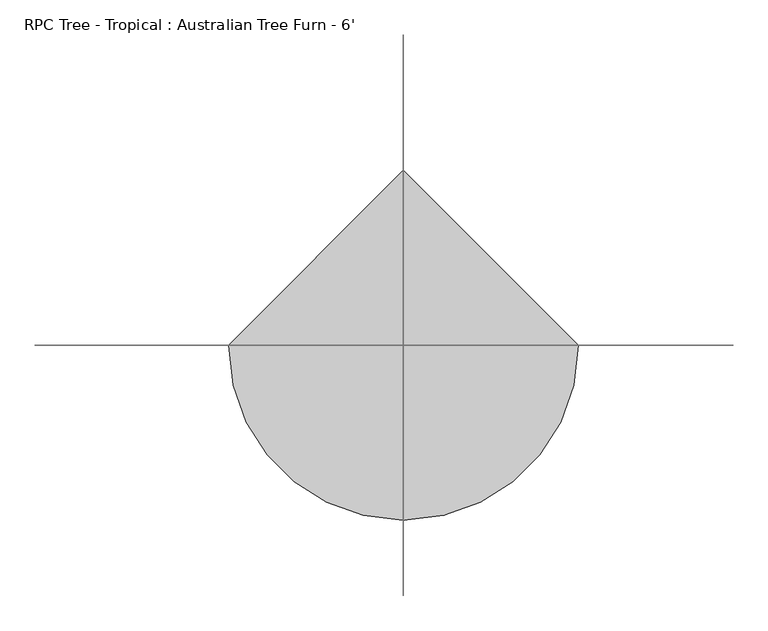
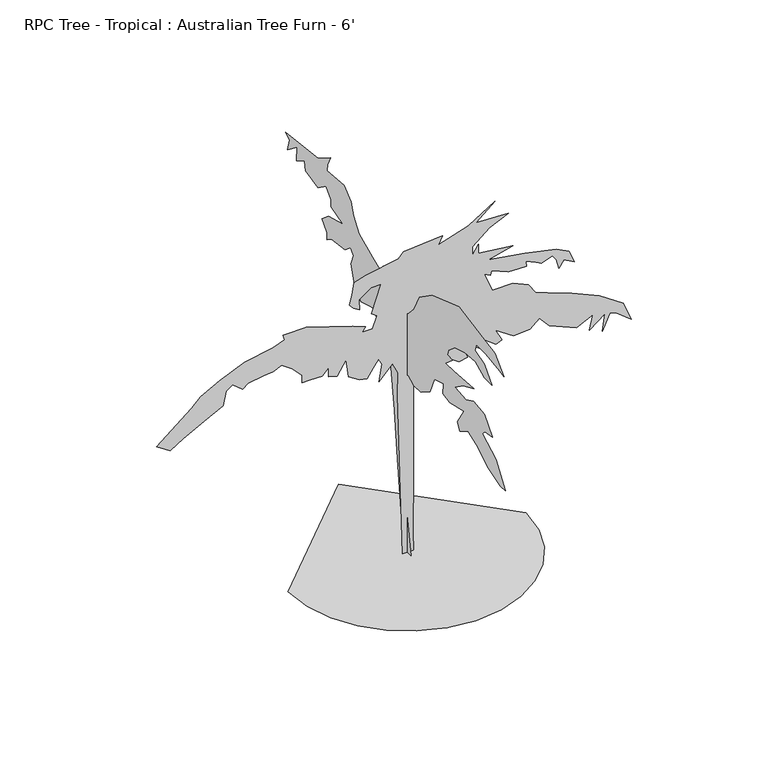
"""IFC4 building model written with IfcOpenShell, lengths in millimetres: geographic element geometry, RPC Tree - Tropical : Australian Tree Furn - 6'."""

from ifc_helpers import new_model, si_unit, origin, place, context, project, spatial, triangles, source, transform, mapped, element, save


def rpc_tree_tropical_australian_tree_furn_6_77f1a640(model_context):
    return source(origin(), model_context, "Body", "Tessellation", [
        triangles([(-639.0365753, 0.0, 0.0007159), (-622.1405136, -146.4247652, 0.0007159), (-574.0277527, -280.8912123, 0.0007159), (-498.5465315, -399.5499215, 0.0007159), (-399.5499215, -498.5465315, 0.0007159), (-280.8912123, -574.0277527, 0.0007159), (-146.4247652, -622.1405136, 0.0007159), (2.79e-05, -639.0365753, 0.0007159), (146.4247652, -622.1429844, 0.0007159), (280.8912123, -574.0277527, 0.0007159), (399.5499215, -498.5465315, 0.0007159), (498.5465315, -399.5499215, 0.0007159), (574.0277527, -280.8912123, 0.0007159), (622.1405136, -146.4247652, 0.0007159), (639.0365753, 5.59e-05, 0.0007159), (-8.38e-05, 639.0365753, 0.0007159), (470.2991641, -3.5e-05, 1828.8014534), (368.5593713, -2.98e-05, 1741.5955845), (542.9711454, -2.94e-05, 1734.3285862), (441.231389, -2.66e-05, 1687.0922253), (350.3907492, -2.2e-05, 1610.7880165), (350.3907492, -1.92e-05, 1563.5516556), (383.0932589, -2.22e-05, 1614.4202076), (383.0932589, -1.92e-05, 1563.5516556), (568.4067295, -1.79e-05, 1541.750806), (437.5966181, -1.59e-05, 1509.0482964), (633.8092781, -1.4e-05, 1476.3456413), (800.9540903, -1.18e-05, 1440.0109406), (869.9913008, -9.7e-06, 1403.673769), (899.0591486, -5.5e-06, 1334.6364132), (840.9235256, -7.5e-06, 1367.3389229), (815.4879416, -5.1e-06, 1327.3695602), (800.9540903, -8.4e-06, 1381.8729195), (779.1532408, -1.01e-05, 1410.9406219), (721.015147, -8.8e-06, 1389.1397724), (691.9473719, -9.7e-06, 1403.673769), (637.4440126, -1.12e-05, 1429.1092804), (641.0762037, -9.4e-06, 1400.0414326), (597.4745047, -9.4e-06, 1400.0414326), (542.9711454, -9.7e-06, 1403.673769), (452.1330491, -1.18e-05, 1440.0109406), (448.4983146, -1.03e-05, 1414.5754292), (415.7958049, -1.14e-05, 1432.7440876), (459.4000111, -5.1e-06, 1327.3695602), (568.4067295, -5.1e-06, 1327.3695602), (651.9778639, -2.9e-06, 1291.0347141), (688.3126373, 3e-07, 1236.5313549), (753.7176567, 1.8e-06, 1211.0958435), (884.5252247, 4.9e-06, 1160.2246754), (1033.5014511, 8.7e-06, 1094.8221268), (1160.6767553, 1.39e-05, 1007.6162579), (1204.2784544, 2.02e-05, 902.2417305), (1120.70732, 1.63e-05, 967.6468225), (1088.0048103, 1.59e-05, 974.9137482), (1048.0353024, 2.11e-05, 887.7078793), (1062.5692263, 1.55e-05, 982.1806738), (978.9980919, 1.94e-05, 916.7781979), (997.1666777, 1.44e-05, 1000.3493322), (909.9608088, 1.7e-05, 956.7450897), (764.6193169, 1.33e-05, 1018.5179907), (710.1159576, 9.6e-06, 1080.2882755), (659.2448622, 1.22e-05, 1036.684033), (572.0389206, 1.26e-05, 1029.4171074), (473.9338986, 8.7e-06, 1094.8221268), (510.2686357, 1.26e-05, 1029.4171074), (477.5660897, 1.35e-05, 1014.8831835), (324.9577085, 6.6e-06, 1131.1569002), (419.4305394, 1.44e-05, 1000.3493322), (284.9882369, 8.7e-06, 1094.8221268), (324.9577085, 1.48e-05, 993.0824066), (277.7212749, 1.52e-05, 985.8154083), (190.5151335, 1.16e-05, 1047.5857658), (88.7756132, 9.6e-06, 1080.2882755), (194.1488688, 1.52e-05, 985.8154083), (30.6385209, 1.11e-05, 1054.8526915), (34.2719928, 1.57e-05, 978.5484827), (34.2719928, 3.32e-05, 684.2282936), (34.2719928, 4.84e-05, 429.8801196), (30.6385209, 6.77e-05, 106.4923825), (34.2719928, 7.35e-05, 0.0013276), (-23.8650472, 7.39e-05, 0.0007003), (-52.9336422, 1.98e-05, 909.5111996), (-49.2999159, 1.22e-05, 1036.684033), (-78.3684632, 8.5e-06, 1098.4543905), (-151.0396997, 1.31e-05, 1022.1501818), (-136.5055487, 7.5e-06, 1116.6229763), (-154.6734259, 5.5e-06, 1149.325486), (-183.7417098, 7.9e-06, 1109.3560507), (-216.4437289, 1.07e-05, 1062.1196171), (-256.4132006, 1.03e-05, 1069.3865427), (-314.5512943, 8.1e-06, 1105.7213161), (-329.0852182, 2e-06, 1207.461109), (-376.3216155, 6.6e-06, 1131.1569002), (-423.5580491, 5.7e-06, 1145.6907515), (-423.5580491, 2.7e-06, 1196.5619196), (-456.2580153, 4.9e-06, 1160.2246754), (-518.0283365, 4.9e-06, 1160.2246754), (-565.2647701, 4.9e-06, 1160.2246754), (-565.2647701, 2.3e-06, 1203.8289179), (-619.7706728, -1e-06, 1258.3322044), (-674.2714886, -3.4e-06, 1298.3017124), (-721.5079222, -2.1e-06, 1276.5008629), (-772.3790903, -1.9e-06, 1272.866201), (-855.9502247, -1e-06, 1258.3322044), (-885.0205433, 3e-07, 1236.5313549), (-939.5239025, -2.3e-06, 1280.133054), (-972.2238688, -8e-07, 1254.6975426), (-990.3925272, 3.8e-06, 1178.3933338), (-1092.13232, 6.8e-06, 1127.5247091), (-1204.773773, 1.05e-05, 1065.7543516), (-1273.8110561, 1.31e-05, 1022.1501818), (-1346.4830738, 1.03e-05, 1069.3865427), (-1157.5373394, 1.2e-06, 1221.9975037), (-1110.3009058, -1.9e-06, 1272.866201), (-1008.561113, -5.1e-06, 1327.3695602), (-874.1188105, -8.6e-06, 1385.5075813), (-721.5079222, -1.03e-05, 1414.5754292), (-659.7375647, -1.16e-05, 1436.3762787), (-667.004563, -1.33e-05, 1465.4439812), (-539.8317295, -1.33e-05, 1465.4439812), (-416.2885437, -1.1e-05, 1425.4770893), (-292.7479377, -8.6e-06, 1385.5075813), (-223.7109271, -7.1e-06, 1360.0720699), (-241.8788043, -5.5e-06, 1334.6364132), (-187.3751907, -5.5e-06, 1334.6364132), (-161.9403697, -9.4e-06, 1400.0414326), (-191.0089079, -1.07e-05, 1421.8422821), (-140.1390206, -1.96e-05, 1570.8185085), (-194.6423889, -1.96e-05, 1570.8185085), (-260.0454098, -1.68e-05, 1523.5821476), (-256.4132006, -1.33e-05, 1465.4439812), (-289.1157284, -1.46e-05, 1487.2474468), (-310.9165598, -1.62e-05, 1512.6804874), (-296.3826722, -1.94e-05, 1567.1838467), (-285.4809939, -2.31e-05, 1628.956675), (-220.0774642, -2.44e-05, 1650.7575245), (-45.666444, -2.63e-05, 1683.4600342), (-20.2313959, -2.81e-05, 1712.5277367), (190.5151335, -2.92e-05, 1730.6963951), (168.7137935, -2.66e-05, 1687.0922253), (328.5898996, -2.96e-05, 1737.9633934), (3.03e-05, -861.8582216, 1549.8330162), (2.4e-05, -733.5424347, 1570.5289913), (2.01e-05, -646.6209961, 1570.5289913), (2.06e-05, -630.0627771, 1529.1370411), (2.54e-05, -721.12437, 1504.3009117), (3.07e-05, -787.3523769, 1425.6574562), (2.76e-05, -716.9866865, 1425.6574562), (2.26e-05, -634.2029314, 1467.0492611), (1.86e-05, -539.0011479, 1458.7689526), (1.52e-05, -443.8018716, 1429.7951397), (1.41e-05, -385.8542459, 1380.1253517), (1.46e-05, -373.4361812, 1347.0113846), (1.68e-05, -423.1059328, 1347.0113846), (1.55e-05, -356.8778895, 1289.0637589), (1.89e-05, -435.5239975, 1293.2039131), (2.69e-05, -621.7848667, 1305.6220505), (2.36e-05, -518.3052092, 1260.089946), (2.19e-05, -443.8018716, 1206.2800037), (2.68e-05, -547.2815291, 1198.0020933), (2.89e-05, -617.6471832, 1231.1161331), (3.37e-05, -716.9866865, 1218.6980684), (3.97e-05, -795.6302147, 1135.9143133), (3.69e-05, -725.2645243, 1123.4987921), (3.66e-05, -700.4309383, 1098.6626627), (4.42e-05, -824.6040276, 1028.2969723), (5.2e-05, -915.6656204, 904.1213396), (4.99e-05, -865.9959051, 899.9836561), (4.34e-05, -745.9604994, 937.2353794), (3.69e-05, -642.4808418, 999.3231594), (3.26e-05, -567.9774679, 1032.4371992), (3.06e-05, -489.3313963, 982.7648678), (2.84e-05, -468.6354575, 1024.1567453), (2.82e-05, -530.7232738, 1123.4987921), (2.33e-05, -398.2697671, 1090.3847523), (2e-05, -332.0443036, 1102.802817), (1.84e-05, -336.1819871, 1160.7504427), (1.55e-05, -253.3997399, 1135.9143133), (1.65e-05, -212.0081348, 1040.715037), (1.44e-05, -129.2246341, 986.9050947), (1.15e-05, -62.9981487, 982.7648678), (8.4e-06, -13.3280768, 1011.7412241), (6.8e-06, 32.2026538, 999.3231594), (4.5e-06, 52.8985925, 1044.8527205), (4.9e-06, 81.8726461, 986.9050947), (7e-06, 86.0118375, 912.3991774), (1.57e-05, 57.0377794, 664.0505281), (2.77e-05, 19.7852431, 316.3597959), (3.93e-05, -34.0238362, 0.0007149), (3.64e-05, 36.3418406, 0.0), (3.07e-05, 52.8985925, 167.3503229), (1.97e-05, 90.1512742, 477.7870791), (1.08e-05, 119.1250779, 734.4162186), (1.5e-06, 156.3777732, 991.0453217), (-4.8e-06, 210.1869524, 1119.3585651), (-7.3e-06, 268.135323, 1119.3585651), (-1.14e-05, 305.3869918, 1198.0020933), (-1.38e-05, 371.6149987, 1181.4464178), (-1.58e-05, 429.5625881, 1160.7504427), (-2.04e-05, 491.6504045, 1222.8382954), (-2.47e-05, 520.6242173, 1322.177726), (-2.55e-05, 499.9282785, 1380.1253517), (-2.76e-05, 528.9020914, 1409.0991646), (-2.86e-05, 578.5718067, 1367.7072144), (-3.37e-05, 702.7474394, 1351.1515388), (-3.47e-05, 744.1393169, 1322.177726), (-3.59e-05, 744.1393169, 1363.5696762), (-3.96e-05, 793.8090322, 1413.2393188), (-3.83e-05, 731.7212523, 1462.9091068), (-3.35e-05, 599.2677455, 1500.1607574), (-3.93e-05, 706.8876663, 1533.2747246), (-4.06e-05, 711.0252771, 1570.5289913), (-4.41e-05, 756.5573816, 1620.1987793), (-4.58e-05, 831.0607555, 1566.3888371), (-5.18e-05, 946.9584778, 1591.2223503), (-5.36e-05, 955.2363155, 1640.8946091), (-5.57e-05, 1029.7422329, 1599.5028042), (-5.79e-05, 1025.602006, 1678.1462597), (-5.98e-05, 1112.525988, 1611.9183254), (-6.09e-05, 1095.9676964, 1674.0061054), (-6.33e-05, 1133.2218904, 1698.8422348), (-5.08e-05, 831.0607555, 1731.9562019), (-4.78e-05, 715.1655041, 1806.4596485), (-4.73e-05, 739.99909, 1752.652177), (-4.64e-05, 748.2795439, 1711.2603722), (-3.97e-05, 586.8496808, 1727.8160477), (-3.52e-05, 520.6242173, 1674.0061054), (-3.23e-05, 499.9282785, 1607.7806419), (-2.78e-05, 446.1183363, 1537.4150242), (-2.05e-05, 321.9452471, 1479.4647823), (-1.04e-05, 143.960199, 1409.0991646), (-1.65e-05, 226.7434454, 1487.7452362), (-9.7e-06, 114.9858956, 1429.7951397), (-2.2e-06, -0.9105653, 1351.1515388), (-1.4e-06, -62.9981487, 1417.3796185), (-2.2e-06, -112.668141, 1516.7190491), (7e-07, -232.7038011, 1599.5028042), (9.2e-06, -481.0535222, 1686.4242428), (2.03e-05, -700.4309383, 1645.0322926), (2.61e-05, -816.3261898, 1624.3363174), (3.23e-05, -899.1099449, 1541.5525623)], [[15, 16, 1], [14, 15, 1], [14, 1, 2], [13, 14, 2], [13, 2, 3], [13, 3, 4], [12, 13, 4], [11, 12, 4], [11, 4, 5], [11, 5, 6], [11, 6, 7], [11, 7, 8], [11, 8, 9], [11, 9, 10], [141, 17, 18], [54, 55, 56], [73, 74, 75], [67, 68, 69], [24, 25, 26], [18, 19, 20], [51, 52, 53], [22, 23, 24], [84, 85, 86], [29, 30, 31], [56, 57, 58], [31, 32, 33], [130, 131, 132], [138, 139, 140], [41, 42, 43], [111, 112, 113], [110, 111, 113], [109, 110, 113], [122, 123, 124], [118, 119, 120], [18, 20, 21], [141, 18, 21], [69, 70, 71], [69, 71, 72], [28, 29, 31], [28, 31, 33], [28, 33, 34], [27, 28, 34], [27, 34, 35], [27, 35, 36], [27, 36, 37], [130, 132, 133], [130, 133, 134], [50, 51, 53], [50, 53, 54], [50, 54, 56], [50, 56, 58], [140, 141, 21], [37, 38, 39], [64, 65, 66], [64, 66, 67], [80, 81, 82], [79, 80, 82], [78, 79, 82], [77, 78, 82], [76, 77, 82], [76, 82, 83], [75, 76, 83], [97, 98, 99], [49, 50, 58], [49, 58, 59], [49, 59, 60], [48, 49, 60], [48, 60, 61], [47, 48, 61], [129, 130, 134], [129, 134, 135], [129, 135, 136], [129, 136, 137], [128, 129, 137], [108, 109, 113], [108, 113, 114], [107, 108, 114], [107, 114, 115], [106, 107, 115], [106, 115, 116], [105, 106, 116], [104, 105, 116], [103, 104, 116], [103, 116, 117], [102, 103, 117], [101, 102, 117], [101, 117, 118], [75, 83, 84], [26, 27, 37], [26, 37, 39], [26, 39, 40], [26, 40, 41], [26, 41, 43], [92, 93, 94], [92, 94, 95], [126, 127, 128], [101, 118, 120], [100, 101, 120], [100, 120, 121], [99, 100, 121], [97, 99, 121], [96, 97, 121], [95, 96, 121], [95, 121, 122], [92, 95, 122], [92, 122, 124], [140, 21, 22], [88, 89, 90], [24, 26, 43], [22, 24, 43], [88, 90, 91], [88, 91, 92], [88, 92, 124], [87, 88, 124], [87, 124, 125], [47, 61, 62], [47, 62, 63], [47, 63, 64], [46, 47, 64], [45, 46, 64], [44, 45, 64], [44, 64, 67], [43, 44, 67], [137, 138, 140], [128, 137, 140], [126, 128, 140], [126, 140, 22], [126, 22, 43], [126, 43, 67], [126, 67, 69], [126, 69, 72], [126, 72, 73], [125, 126, 73], [87, 125, 73], [87, 73, 75], [87, 75, 84], [87, 84, 86], [231, 232, 233], [156, 157, 158], [240, 241, 142], [222, 223, 224], [218, 219, 220], [220, 221, 222], [218, 220, 222], [153, 154, 155], [240, 142, 143], [239, 240, 143], [146, 147, 148], [205, 206, 207], [162, 163, 164], [156, 158, 159], [216, 217, 218], [216, 218, 222], [166, 167, 168], [166, 168, 169], [222, 224, 225], [239, 143, 144], [238, 239, 144], [146, 148, 149], [145, 146, 149], [165, 166, 169], [165, 169, 170], [207, 208, 209], [188, 189, 190], [188, 190, 191], [188, 191, 192], [187, 188, 192], [187, 192, 193], [186, 187, 193], [186, 193, 194], [185, 186, 194], [171, 172, 173], [171, 173, 174], [145, 149, 150], [155, 156, 159], [165, 170, 171], [165, 171, 174], [175, 176, 177], [182, 183, 184], [205, 207, 209], [205, 209, 210], [204, 205, 210], [203, 204, 210], [161, 162, 164], [161, 164, 165], [161, 165, 174], [160, 161, 174], [159, 160, 174], [159, 174, 175], [159, 175, 177], [155, 159, 177], [238, 144, 145], [238, 145, 150], [237, 238, 150], [237, 150, 151], [237, 151, 152], [236, 237, 152], [235, 236, 152], [235, 152, 153], [235, 153, 155], [235, 155, 177], [235, 177, 178], [234, 235, 178], [234, 178, 179], [234, 179, 180], [234, 180, 181], [234, 181, 182], [234, 182, 184], [231, 233, 234], [231, 234, 184], [214, 215, 216], [214, 216, 222], [213, 214, 222], [213, 222, 225], [213, 225, 226], [212, 213, 226], [212, 226, 227], [212, 227, 228], [211, 212, 228], [210, 211, 228], [210, 228, 229], [203, 210, 229], [203, 229, 230], [202, 203, 230], [184, 185, 194], [184, 194, 195], [231, 184, 195], [230, 231, 195], [230, 195, 196], [230, 196, 197], [202, 230, 197], [202, 197, 198], [201, 202, 198], [200, 201, 198], [199, 200, 198]], closed=False),
    ])


if __name__ == "__main__":
    model = new_model("IFC4")
    model_context = context("Model", 3, world=origin())
    ifc_project = project(units=[si_unit("LENGTHUNIT", "METRE", prefix="MILLI")], contexts=[model_context])
    site = spatial("IfcSite", under=ifc_project)
    building = spatial("IfcBuilding", under=site)
    placement = place(None, origin())
    rpc_tree_tropical_australian_tree_furn_6_shape = rpc_tree_tropical_australian_tree_furn_6_77f1a640(model_context)
    element("IfcGeographicElement", 1, ObjectType="RPC Tree - Tropical : Australian Tree Furn - 6'", at=placement, inside=building, context=model_context, shape_type="MappedRepresentation", body=[
        mapped(rpc_tree_tropical_australian_tree_furn_6_shape, transform((0.0, 0.0, 0.0), x_axis=(1.0, 0.0, 0.0), y_axis=(0.0, 1.0, 0.0), z_axis=(0.0, 0.0, 1.0))),
    ])
    save(model, "model.ifc")

# Revit data of these elements
# Type "RPC Tree - Tropical : Australian Tree Furn - 6'"
#   built-in parameter 1005198 = "{2, 15},{39, RPC-16-FVCN-UWG0-AP53-A000-ST1L-LVER-AU},{1, 0},{1, 0},{2, 13},{1, 8},{5, Color},{1, 0},{1, 0},{3, 0.8},{3, 0.8},{3, 0.8},{1, 8},{7, BBoxMin},{1, 0},{1, 0},{1, 0},{1, 0},{1, 0},{1, 8},{7, BBoxMax},{1, 0},{1, 0},{1, 0},{1, 0},{1, 0},{2, 11},{9, RPCTypeId},{1, 0},{1, 0},{39, RPC-16-FVCN-UWG0-AP53-A000-ST1L-LVER-AU},{1, 6},{14, RPCPlantHeight},{1, 0},{1, 0},{1, 6},{2, 11},{7, keyword},{1, 0},{1, 0},{35, :RPCs:Trees [Tropical]:Geometry:RPC},{2, 11},{8, category},{1, 0},{1, 0},{16, Trees [Tropical]},{2, 11},{12, LocalizedUID},{1, 0},{1, 0},{20, Australian Tree Fern},{2, 14},{6, Height},{1, 0},{1, 0},{1, 6},{1, 2},{16, Cast Reflections},{1, 0},{1, 0},{1, 0},{1, 2},{12, Cast Shadows},{1, 0},{1, 0},{1, 1},{1, 2},{9, Lock View},{1, 0},{1, 0},{1, 0},{1, 4},{5, ViewC},{1, 0},{1, 0},{1, 0},{21, assetlibrary_base.fbx},{1, 5},"
#   built-in parameter 1005195 = "RPC-16-FVCN-UWG0-AP53-A000-ST1L-LVER-AU"
#   Type Comments = "Australian Tree Furn"
#   Assembly Code = "G2050500"
#   Height = 6' - 0"
#   Plan Symbol = element 387627
#   Default Elevation = 0
